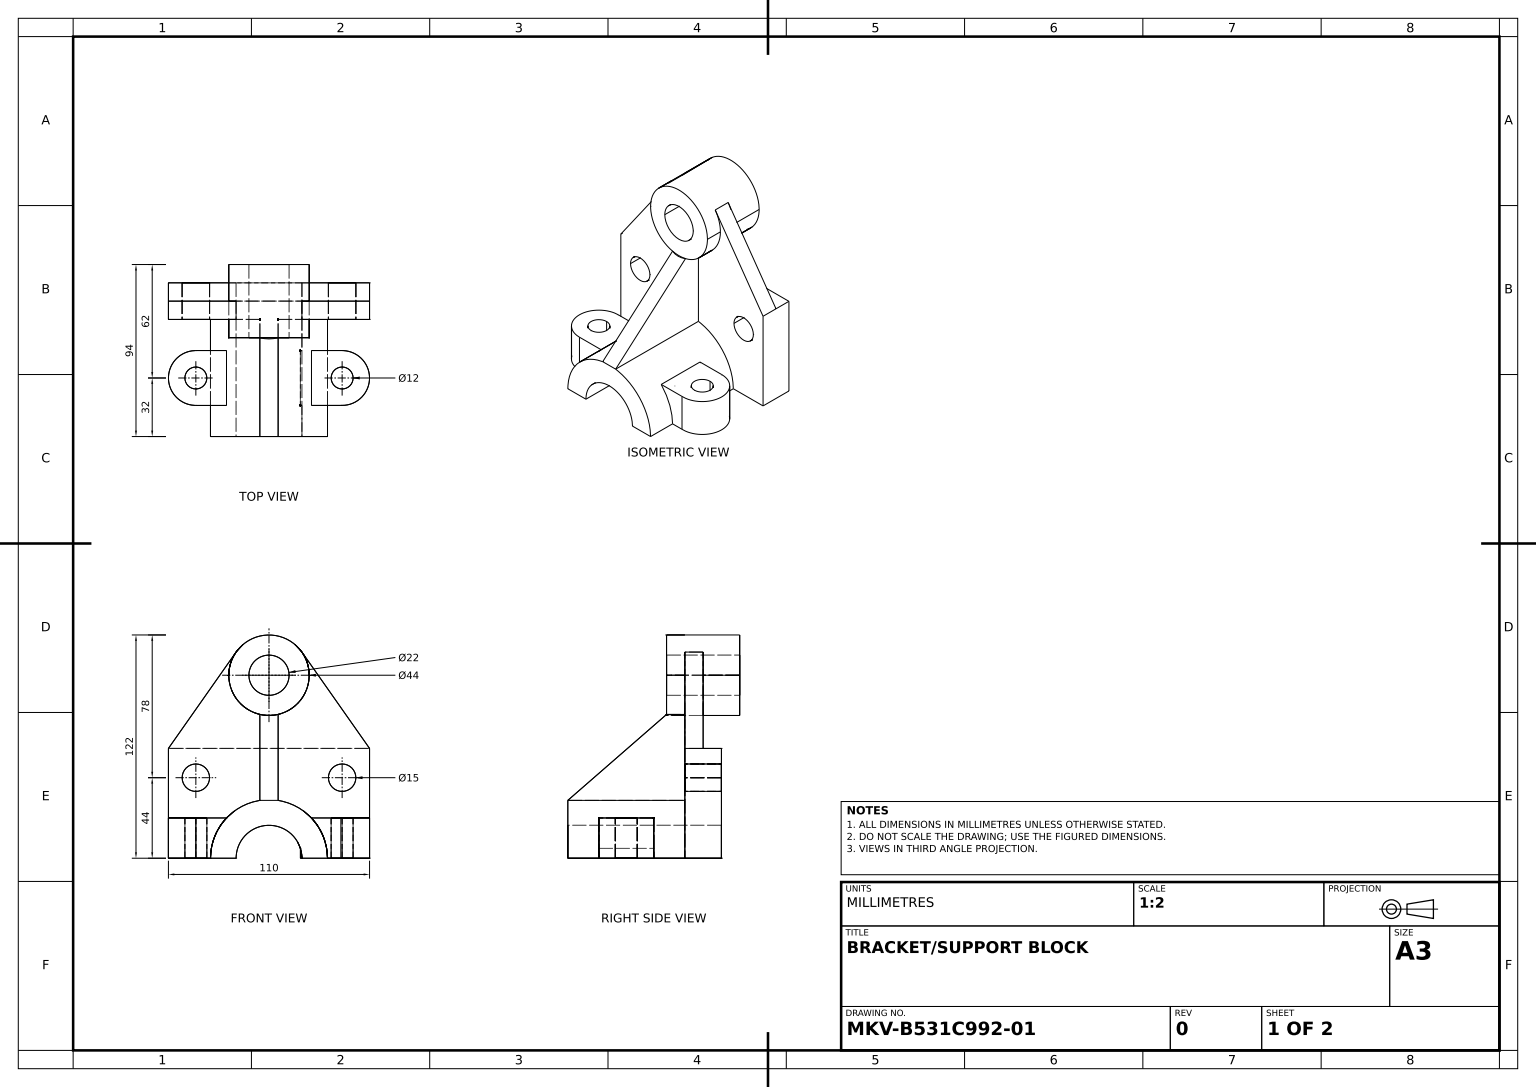
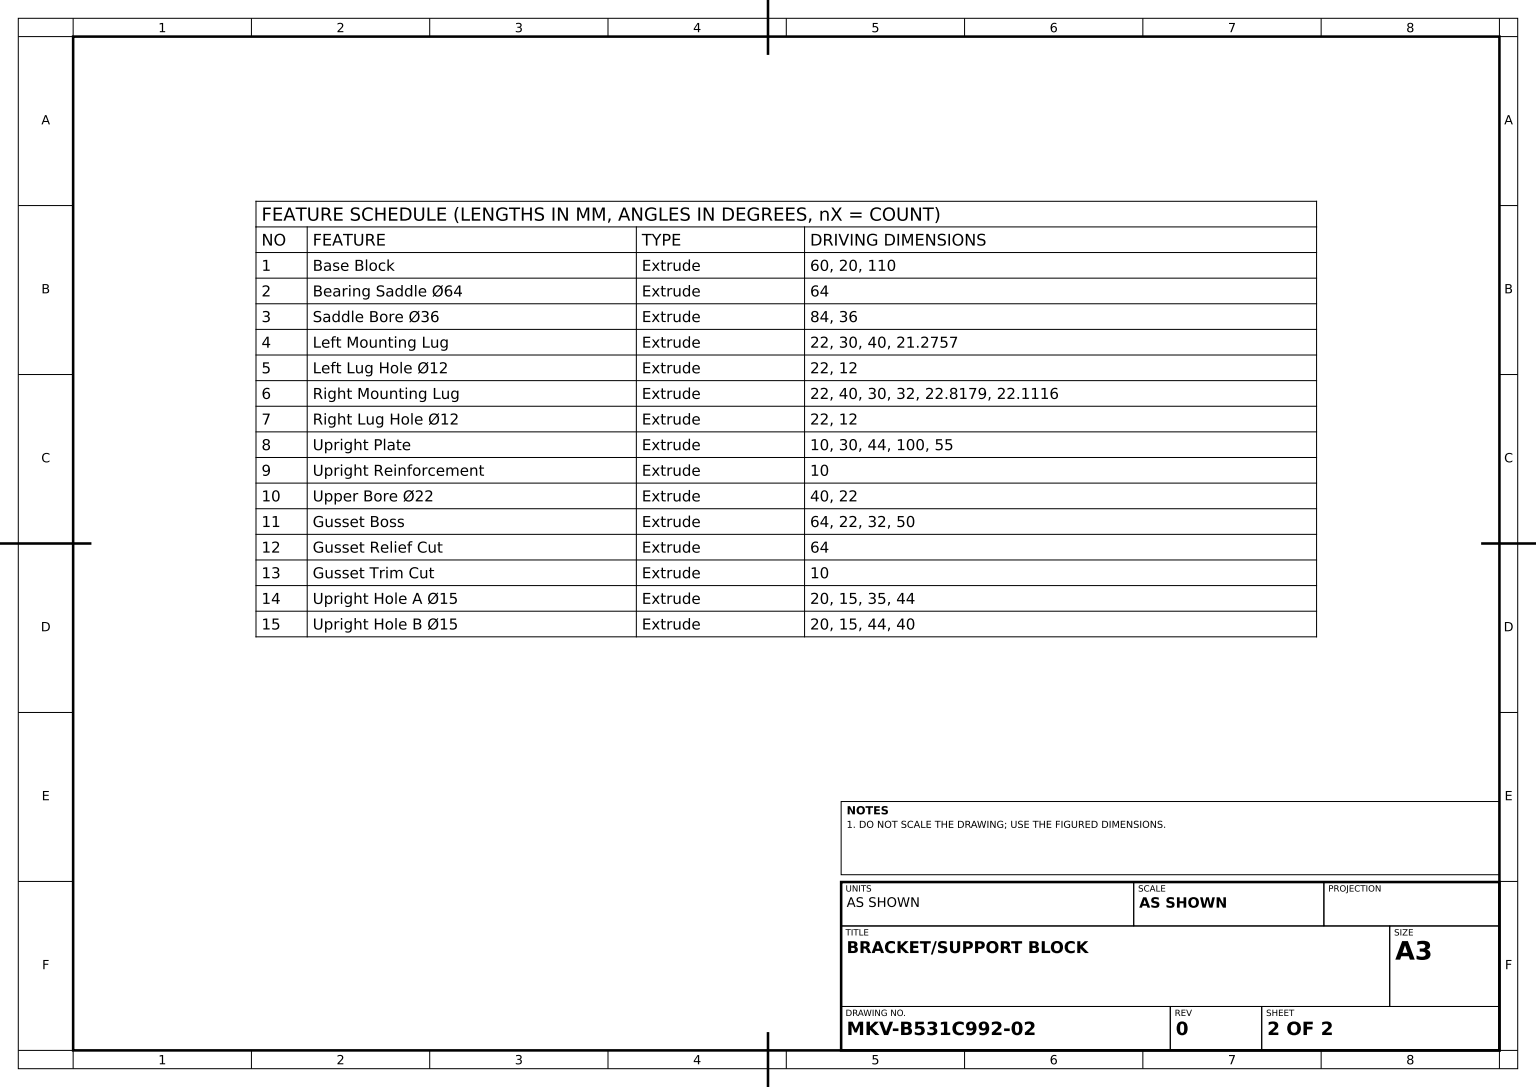
SolidWorks part; units mm, degrees
material "Plain Carbon Steel"
ref_plane "Front Plane" through (0, 0, 0) normal (0, 0, 1) x (1, 0, 0)
ref_plane "Top Plane" through (0, 0, 0) normal (0, 1, 0) x (1, 0, 0)
ref_plane "Right Plane" through (0, 0, 0) normal (1, 0, 0) x (0, 0, -1)
sketch "Base Block Sketch" plane through (0, 0, 0) normal (0, 1, 0) x (1, 0, 0)
  line L0 (-55, 20) -> (55, 20)
  line L1 (55, 20) -> (55, 0)
  line L2 (55, 0) -> (-55, 0)
  line L3 (-55, 0) -> (-55, 20)
  point P2 (0, 0)
  dimension "D1" = 20
  dimension "D2" = 110
extrude "Base Block" add sketch "Base Block Sketch" along normal blind 60
sketch "Bearing Saddle Sketch" plane through (0, 0, 0) normal (0, 0, 1) x (1, 0, 0)
  line L0 (-32, 0) -> (32, 0)
  arc A0 (32, 0) -> (-32, 0) centre (0, 0) ccw
  dimension "D1" = 64
extrude "Bearing Saddle Ø64" add sketch "Bearing Saddle Sketch" along normal blind 64
sketch "Saddle Bore Sketch" plane through (0, 0, 64) normal (0, 0, 1) x (1, 0, 0)
  line L0 (-18, 0) -> (18, 0)
  arc A0 (18, 0) -> (-18, 0) centre (0, 0) ccw
  dimension "D1" = 36
extrude "Saddle Bore Ø36" cut sketch "Saddle Bore Sketch" against normal blind 84
sketch "Left Lug Sketch" plane through (0, 0, 0) normal (0, 1, 0) x (1, 0, 0)
  line L0 (-32, -32) -> (-40, -32) construction
  line L1 (-32, -64) -> (-32, 0) construction
  line L2 (-40, -17) -> (-18.7243, -17)
  line L3 (-18.7243, -17) -> (-18.7243, -47)
  line L4 (-18.7243, -47) -> (-40, -47)
  arc A0 (-40, -17) -> (-40, -47) centre (-40, -32) ccw
  dimension "D1" = 30
  dimension "D2" = 40
  dimension "D3" = 21.2757
extrude "Left Mounting Lug" add sketch "Left Lug Sketch" along normal blind 22
sketch "Left Lug Hole Sketch" plane through (0, 22, 0) normal (0, 1, 0) x (1, 0, 0)
  circle A0 centre (-40, -32) radius 6
  dimension "D1" = 12
extrude "Left Lug Hole Ø12" cut sketch "Left Lug Hole Sketch" against normal blind 22
sketch "Right Lug Sketch" plane through (0, 0, 0) normal (0, 1, 0) x (1, 0, 0)
  line L0 (0, -32) -> (40, -32) construction
  line L1 (-32, -64) -> (32, -64) construction
  line L2 (40, -17) -> (17.1821, -17)
  line L3 (17.1821, -17) -> (17.1821, -47)
  line L4 (17.1821, -47) -> (39.2937, -46.9834)
  arc A0 (39.2937, -46.9834) -> (40, -17) centre (40, -32) ccw
  dimension "D2" = 30
  dimension "D1" = 40
  dimension "D3" = 32
  dimension "D4" = 22.8179
  dimension "D5" = 30
  dimension "D6" = 22.1116
extrude "Right Mounting Lug" add sketch "Right Lug Sketch" along normal blind 22
sketch "Right Lug Hole Sketch" plane through (0, 22, 0) normal (0, 1, 0) x (1, 0, 0)
  circle A0 centre (40, -32) radius 6
  dimension "D1" = 12
extrude "Right Lug Hole Ø12" cut sketch "Right Lug Hole Sketch" against normal blind 22
sketch "Upright Plate Sketch" plane through (0, 0, 0) normal (0, 0, 1) x (1, 0, 0)
  line L0 (55, 60) -> (55, 0) construction
  circle A0 centre (0, 100) radius 22
  dimension "D1" = 44
  dimension "D2" = 100
  dimension "D3" = 55
extrude "Upright Plate" add sketch "Upright Plate Sketch" along normal blind 10 and the other way blind 30 separate body
sketch "Upright Reinforcement Sketch" plane through (0, 0, 0) normal (0, 0, 1) x (1, 0, 0)
  line L0 (-55, 60) -> (-17.9997, 112.6496)
  line L1 (55, 60) -> (17.9997, 112.6496)
  line L2 (-55, 60) -> (55, 60)
  circle A0 centre (0, 100) radius 22 construction
  arc A1 (-17.9997, 112.6496) -> (17.9997, 112.6496) centre (0, 100) ccw
extrude "Upright Reinforcement" add sketch "Upright Reinforcement Sketch" against normal blind 10
sketch "Upper Bore Sketch" plane through (0, 0, 10) normal (0, 0, 1) x (1, 0, 0)
  circle A0 centre (0, 100) radius 11
  dimension "D1" = 22
extrude "Upper Bore Ø22" cut sketch "Upper Bore Sketch" against normal blind 40
sketch "Gusset Boss Sketch" plane through (0, 0, 0) normal (0, 0, 1) x (1, 0, 0)
  line L0 (55, 60) -> (55, 0) construction
  line L1 (-5, 78.5757) -> (-5, 31.607)
  line L2 (5, 78.5757) -> (5, 31.607)
  arc A0 (-5, 78.5757) -> (5, 78.5757) centre (0, 100) ccw
  arc A1 (5, 31.607) -> (-5, 31.607) centre (0, 0) ccw
  dimension "D1" = 22
  dimension "D2" = 32
  dimension "D3" = 50
extrude "Gusset Boss" add sketch "Gusset Boss Sketch" along normal blind 64
sketch "Gusset Relief Sketch" plane through (0, 0, 0) normal (1, 0, 0) x (0, 0, -1)
  line L0 (-10, 78.5757) -> (-64, 31.607)
  line L1 (-64, 31.607) -> (-64, 78.5757)
  line L2 (-64, 78.5757) -> (-10, 78.5757)
extrude "Gusset Relief Cut" cut sketch "Gusset Relief Sketch" against normal blind 64
sketch "Gusset Trim Sketch" plane through (0, 0, 0) normal (-1, 0, 0) x (0, 0, 1)
  line L0 (10, 78.5757) -> (64, 31.607)
  line L1 (64, 31.607) -> (64, 78.5757)
  line L2 (64, 78.5757) -> (10, 78.5757)
extrude "Gusset Trim Cut" cut sketch "Gusset Trim Sketch" against normal blind 10
sketch "Upright Hole A Sketch" plane through (0, 0, 0) normal (0, 0, 1) x (1, 0, 0)
  line L0 (5, 31.607) -> (5, 78.5757) construction
  circle A0 centre (40, 44) radius 7.5
  dimension "D1" = 15
  dimension "D2" = 35
  dimension "D3" = 44
extrude "Upright Hole A Ø15" cut sketch "Upright Hole A Sketch" against normal blind 20
sketch "Upright Hole B Sketch" plane through (0, 0, 0) normal (0, 0, 1) x (1, 0, 0)
  circle A0 centre (-40, 44) radius 7.5
  dimension "D1" = 15
  dimension "D2" = 44
  dimension "D3" = 40
extrude "Upright Hole B Ø15" cut sketch "Upright Hole B Sketch" against normal blind 20
